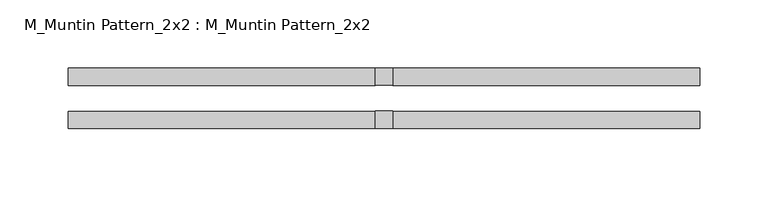
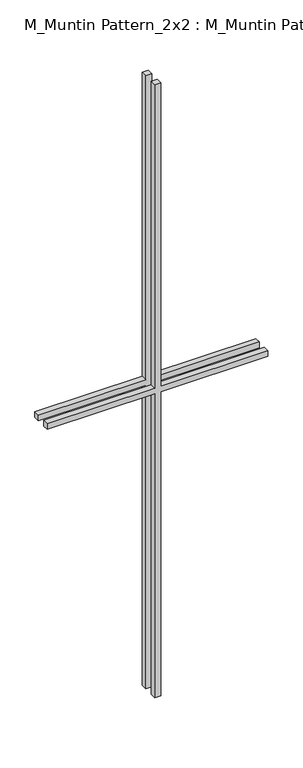
"""IFC4 building model written with IfcOpenShell, lengths in millimetres: proxy geometry, M_Muntin Pattern_2x2 : M_Muntin Pattern_2x2."""

from ifc_helpers import new_model, si_unit, frame, origin, place, context, project, spatial, polyline, outline, extrude, source, transform, mapped, element, save


def m_muntin_pattern_2x2_m_muntin_pattern_2x2_d4676b39(model_context):
    return source(origin(), model_context, "Body", "SweptSolid", [
        extrude(outline(polyline([(686.5, -6.35), (686.5, -231.7375), (673.8, -231.7375), (673.8, -6.35), (0.0, -6.35), (0.0, 6.35), (673.8, 6.35), (673.8, 231.7375), (686.5, 231.7375), (686.5, 6.35), (1360.3, 6.35), (1360.3, -6.35), (686.5, -6.35)])), frame((0.0, 9.525, 0.0), z_axis=(0.0, 1.0, 0.0), x_axis=(0.0, 0.0, 1.0)), (0.0, 0.0, 1.0), 12.7),
        extrude(outline(polyline([(686.5, -6.35), (686.5, -231.7375), (673.8, -231.7375), (673.8, -6.35), (0.0, -6.35), (0.0, 6.35), (673.8, 6.35), (673.8, 231.7375), (686.5, 231.7375), (686.5, 6.35), (1360.3, 6.35), (1360.3, -6.35), (686.5, -6.35)])), frame((0.0, -22.225, 0.0), z_axis=(0.0, 1.0, 0.0), x_axis=(0.0, 0.0, 1.0)), (0.0, 0.0, 1.0), 12.7),
    ])


if __name__ == "__main__":
    model = new_model("IFC4")
    model_context = context("Model", 3, world=origin())
    ifc_project = project(units=[si_unit("LENGTHUNIT", "METRE", prefix="MILLI")], contexts=[model_context])
    site = spatial("IfcSite", under=ifc_project)
    building = spatial("IfcBuilding", under=site)
    placement = place(None, origin())
    m_muntin_pattern_2x2_m_muntin_pattern_2x2_shape = m_muntin_pattern_2x2_m_muntin_pattern_2x2_d4676b39(model_context)
    element("IfcBuildingElementProxy", 1, Name="M_Muntin Pattern_2x2 : M_Muntin Pattern_2x2", ObjectType="M_Muntin Pattern_2x2 : M_Muntin Pattern_2x2", at=placement, inside=building, context=model_context, shape_type="MappedRepresentation", body=[
        mapped(m_muntin_pattern_2x2_m_muntin_pattern_2x2_shape, transform((0.0, 0.0, 0.0), x_axis=(1.0, 0.0, 0.0), y_axis=(0.0, 1.0, 0.0), z_axis=(0.0, 0.0, 1.0))),
    ])
    save(model, "model.ifc")

# Revit data of these elements
# Type "M_Muntin Pattern_2x2 : M_Muntin Pattern_2x2"
#   Width [instance default] = 3.937008 ft
#   Thickness = 0.041667 ft
#   Height [instance default] = 3.937008 ft
#   Distance = 0.0625 ft
#   Interior Material [instance default] = none
#   Exterior Material [instance default] = none
#   Default Elevation = 0
# Element 1 (IfcBuildingElementProxy, "M_Muntin Pattern_2x2 : M_Muntin Pattern_2x2")
#   Width = 1.520587 ft
#   Height = 4.462927 ft
#   Interior Material = Wood - Stained
#   Exterior Material = Clad - White
#   Materials on its faces: "Clad - White", "Wood - Stained"
# Materials
#   "Clad - White": class "Wood", colour RGB 242 242 238, transparency 0, Cost = 0
#   "Wood - Stained": class "Wood", colour RGB 224 178 126, transparency 0, Cost = 0
